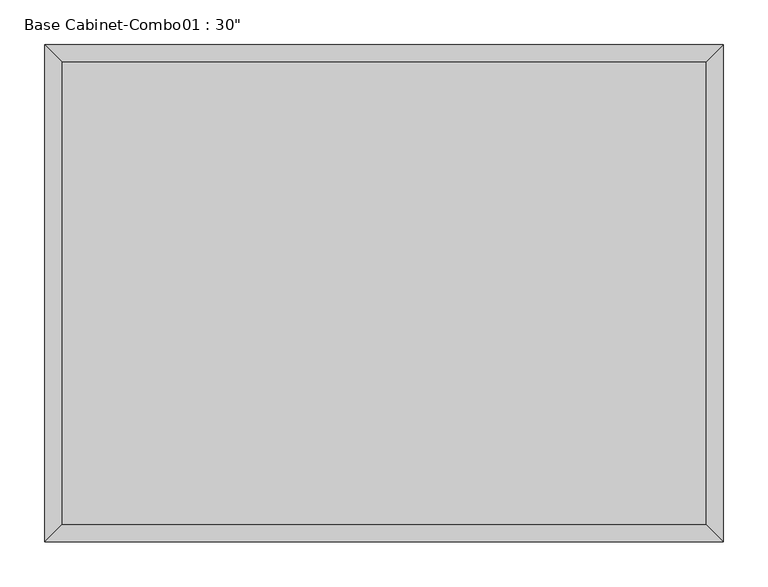
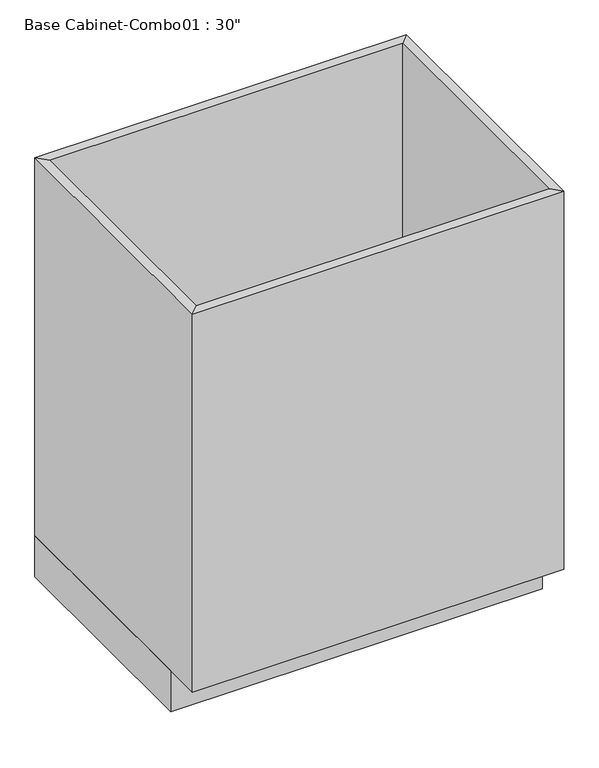
"""IFC4 building model written with IfcOpenShell, lengths in millimetres: furniture geometry."""

from ifc_helpers import new_model, si_unit, frame, origin, origin_with_axes, place, context, project, spatial, polyline, outline, extrude, faceted_brep, source, transform, mapped, element, save


def furniture_f87f75a4(model_context):
    return source(origin(), model_context, "Body", "SolidModel", [
        extrude(outline(polyline([(399.7377049, 0.0), (399.7377049, -482.6), (-362.2622951, -482.6), (-362.2622951, 0.0), (399.7377049, 0.0)])), origin_with_axes(), (0.0, 0.0, 1.0), 88.9),
        faceted_brep([(380.6877049, -539.75, 908.05), (380.6877049, -539.75, 88.9), (-343.2122951, -539.75, 88.9), (-343.2122951, -539.75, 908.05), (399.7377049, -558.8, 908.05), (-362.2622951, -558.8, 908.05), (399.7377049, -558.8, 88.9), (-362.2622951, -558.8, 88.9), (-343.2122951, -19.05, 88.9), (-343.2122951, -19.05, 908.05), (-362.2622951, 0.0, 908.05), (-362.2622951, 0.0, 88.9), (380.6877049, -19.05, 88.9), (380.6877049, -19.05, 908.05), (399.7377049, 0.0, 908.05), (399.7377049, 0.0, 88.9)], [[[0, 1, 2, 3]], [[4, 0, 3, 5]], [[6, 4, 5, 7]], [[1, 6, 7, 2]], [[3, 2, 8, 9]], [[5, 3, 9, 10]], [[7, 5, 10, 11]], [[2, 7, 11, 8]], [[9, 8, 12, 13]], [[10, 9, 13, 14]], [[11, 10, 14, 15]], [[8, 11, 15, 12]], [[13, 12, 1, 0]], [[14, 13, 0, 4]], [[15, 14, 4, 6]], [[12, 15, 6, 1]]]),
        extrude(outline(polyline([(380.6877049, -19.05), (380.6877049, -539.75), (-343.2122951, -539.75), (-343.2122951, -19.05), (380.6877049, -19.05)])), frame((0.0, 0.0, 88.9), z_axis=(0.0, 0.0, 1.0), x_axis=(1.0, 0.0, 0.0)), (0.0, 0.0, 1.0), 19.05),
    ])


if __name__ == "__main__":
    model = new_model("IFC4")
    model_context = context("Model", 3, world=origin())
    ifc_project = project(units=[si_unit("LENGTHUNIT", "METRE", prefix="MILLI")], contexts=[model_context])
    site = spatial("IfcSite", under=ifc_project)
    building = spatial("IfcBuilding", under=site)
    placement = place(None, origin())
    furniture_shape = furniture_f87f75a4(model_context)
    element("IfcFurniture", 1, ObjectType="Base Cabinet-Combo01 : 30\"", at=placement, inside=building, context=model_context, shape_type="MappedRepresentation", body=[
        mapped(furniture_shape, transform((0.0, 0.0, 0.0), x_axis=(1.0, 0.0, 0.0), y_axis=(0.0, 1.0, 0.0), z_axis=(0.0, 0.0, 1.0))),
    ])
    save(model, "model.ifc")

# Revit data of these elements
# Type "Base Cabinet-Combo01 : 30\""
#   Depth = 1.833333 ft
#   Height = 2.979167 ft
#   Toe Depth = 0.25 ft
#   Toe Height = 0.291667 ft
#   Width = 2.5 ft
#   Default Elevation = 0
# Element 1 (IfcFurniture, "Base Cabinet-Combo01 : 30\"")
#   Materials on its faces: "Cabinet"
# Materials
#   "Cabinet": colour RGB 204 122 2, transparency 0
